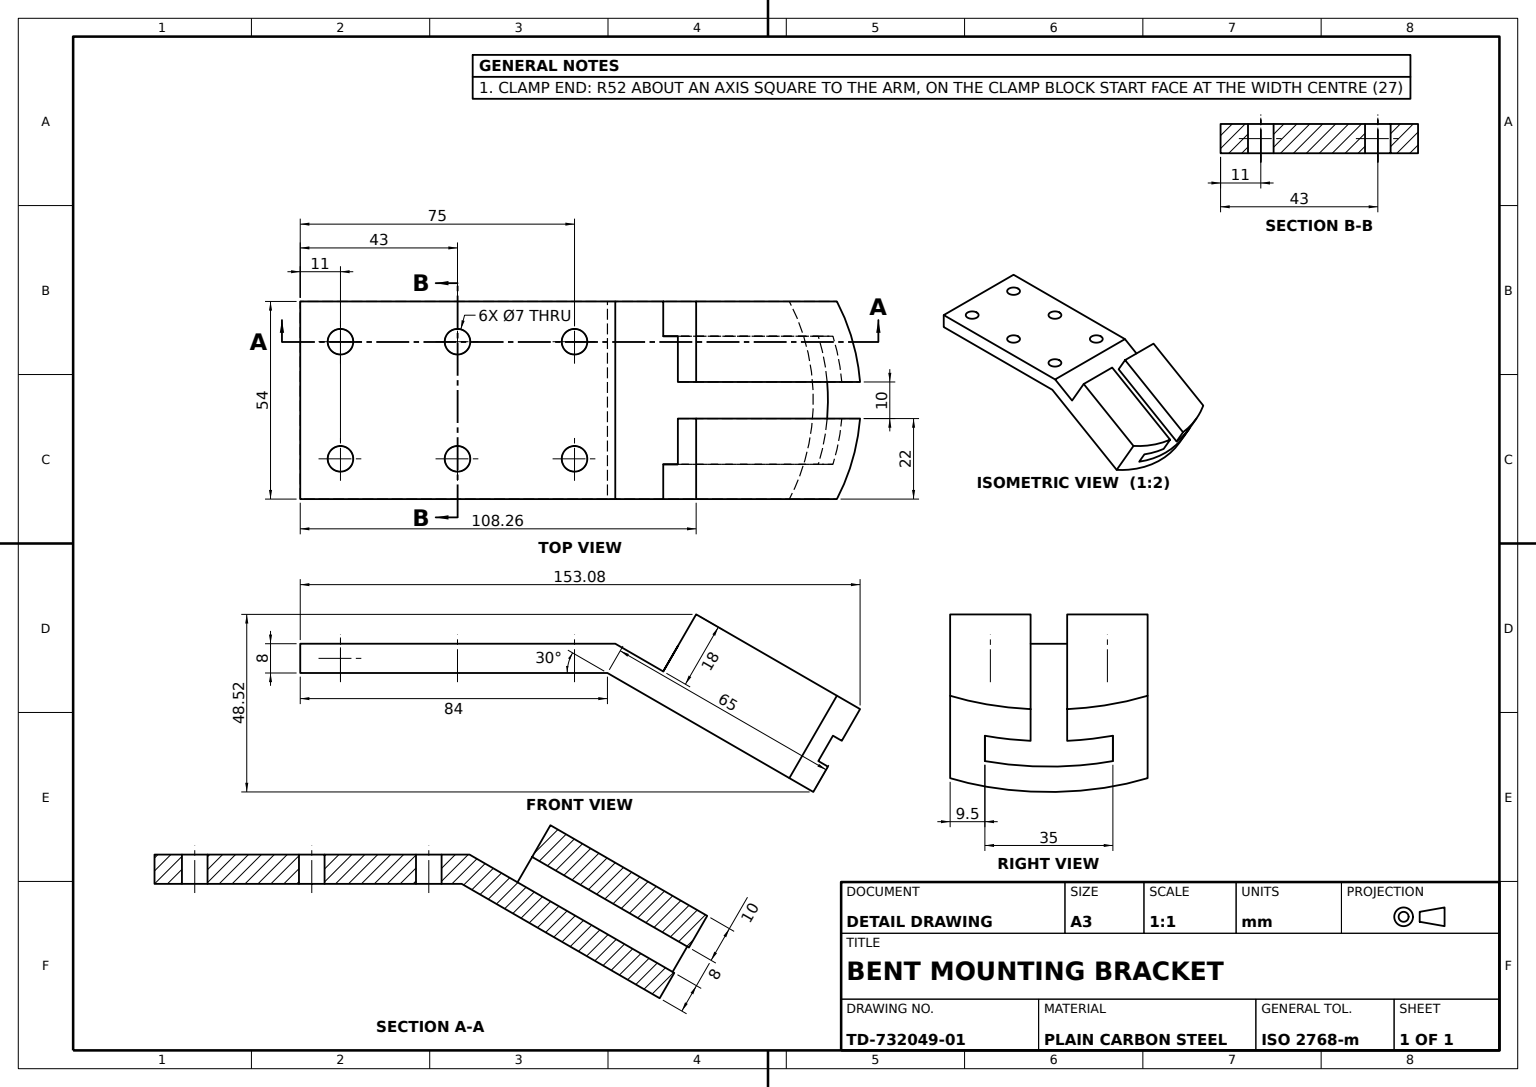
SolidWorks part; units mm, degrees
material "Plain Carbon Steel"
ref_plane "Front Plane" through (0, 0, 0) normal (0, 0, 1) x (1, 0, 0)
ref_plane "Top Plane" through (0, 0, 0) normal (0, 1, 0) x (1, 0, 0)
ref_plane "Right Plane" through (0, 0, 0) normal (1, 0, 0) x (0, 0, -1)
sketch "Bracket Profile Sketch" plane through (0, 0, 0) normal (0, 0, 1) x (1, 0, 0)
  line L0 (84, 0) -> (140.2917, -32.5)
  line L1 (0, 0) -> (84, 0)
  line L2 (0, 0) -> (0, 8)
  line L3 (0, 8) -> (86.1436, 8)
  line L5 (140.2917, -32.5) -> (153.2917, -9.9833)
  line L6 (153.2917, -9.9833) -> (108.2583, 16.0167)
  line L7 (108.2583, 16.0167) -> (99.2583, 0.4282)
  line L8 (99.2583, 0.4282) -> (86.1436, 8)
  line L9 (86.1436, 8) -> (99.2583, 0.4282)
  dimension "D1" = 84
  dimension "D2" = 65
  dimension "D3" = 8
  dimension "D4" = 30
  dimension "D5" = 26
  dimension "D6" = 8
  dimension "D7" = 52
extrude "Bracket Body" add sketch "Bracket Profile Sketch" along normal mid plane 54 contours L7 L8 L3 L2 L1 L0 L5 L6
sketch "Clamp Slot Sketch" plane through (119.2917, -68.8731, 0) normal (0.866, -0.5, 0) x (0, 0, -1)
  line L0 (-27, 68) -> (27, 68) construction
  line L3 (-17.5, 50) -> (17.5, 50)
  line L9 (-17.5, 58) -> (-17.5, 50)
  line L13 (17.5, 58) -> (17.5, 50)
  line L14 (-17.5, 58) -> (-5, 58)
  line L21 (-5, 68) -> (-5, 58)
  line L24 (17.5, 58) -> (5, 58)
  line L25 (5, 68) -> (5, 58)
  line L28 (-5, 68) -> (5, 68)
  dimension "D1" = 9.5
  dimension "D2" = 10
  dimension "D3" = 35
  dimension "D4" = 18
  dimension "D6" = 10
extrude "Clamp Slot" cut sketch "Clamp Slot Sketch" against normal blind 54
sketch "Clamp End Trim Sketch" plane through (34, 58.8897, 0) normal (0.5, 0.866, 0) x (0.866, -0.5, 0)
  line L1 (85.7461, 5) -> (85.7461, 27) construction
  line L2 (130.1871, 27) -> (186.7106, 27)
  line L3 (186.7106, 27) -> (186.7106, -27)
  line L4 (186.7106, -27) -> (130.1871, -27)
  arc A0 (130.1871, -27) -> (130.1871, 27) centre (85.7461, 0) ccw
  dimension "D1" = 52
  dimension "D2" = 44.441
  dimension "D3" = 100.9644
  dimension "D4" = 27
extrude "Clamp End Trim" cut sketch "Clamp End Trim Sketch" against normal blind 54
sketch "Mounting Holes Sketch" plane through (0, 8, 0) normal (0, 1, 0) x (1, 0, 0)
  line L0 (0, 27) -> (86.1436, 27) construction
  line L1 (0, -27) -> (0, 27) construction
  circle A0 centre (11, 16) radius 3.5
  circle A1 centre (43, 16) radius 3.5
  circle A2 centre (75, 16) radius 3.5
  circle A3 centre (11, -16) radius 3.5
  circle A4 centre (43, -16) radius 3.5
  circle A5 centre (75, -16) radius 3.5
  dimension "D1" = 7
  dimension "D2" = 11
  dimension "D3" = 11
  dimension "D6" = 43
  dimension "D7" = 43
  dimension "D4" = 3
  dimension "D5" = 2
extrude "Mounting Holes 6xØ7" cut sketch "Mounting Holes Sketch" against normal blind 54
